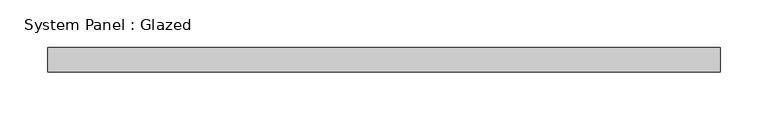
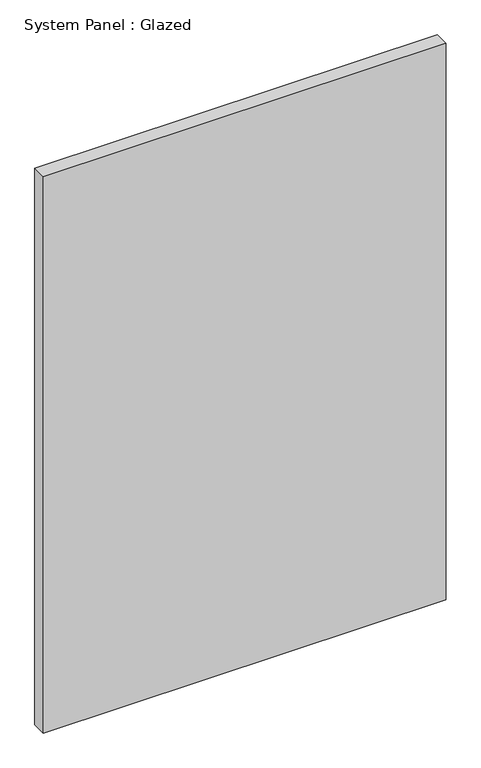
"""IFC4 building model written with IfcOpenShell, lengths in millimetres: plate geometry, System Panel : Glazed."""

from ifc_helpers import new_model, si_unit, origin, origin_with_axes, place, context, project, spatial, polyline, outline, extrude, source, transform, mapped, element, save


def system_panel_glazed_8af8589b(model_context):
    return source(origin(), model_context, "Body", "SweptSolid", [
        extrude(outline(polyline([(350.3083333, 19.05), (-350.3083333, 19.05), (-350.3083333, 44.45), (350.3083333, 44.45), (350.3083333, 19.05)])), origin_with_axes(), (0.0, 0.0, 1.0), 1022.35),
    ])


if __name__ == "__main__":
    model = new_model("IFC4")
    model_context = context("Model", 3, world=origin())
    ifc_project = project(units=[si_unit("LENGTHUNIT", "METRE", prefix="MILLI")], contexts=[model_context])
    site = spatial("IfcSite", under=ifc_project)
    building = spatial("IfcBuilding", under=site)
    placement = place(None, origin())
    system_panel_glazed_shape = system_panel_glazed_8af8589b(model_context)
    element("IfcPlate", 1, ObjectType="System Panel : Glazed", at=placement, inside=building, context=model_context, shape_type="MappedRepresentation", body=[
        mapped(system_panel_glazed_shape, transform((0.0, 0.0, 0.0), x_axis=(1.0, 0.0, 0.0), y_axis=(0.0, 1.0, 0.0), z_axis=(0.0, 0.0, 1.0))),
    ])
    save(model, "model.ifc")

# Revit data of these elements
# Type "System Panel : Glazed"
#   Construction Type Id = "GSP4R"
#   Analytic Construction = "1/8 in Pilkington single glazing"
#   Visual Light Transmittance = 0.9
#   Solar Heat Gain Coefficient = 0.86
#   Heat Transfer Coefficient (U) = 1.18115 BTU/(h·ft²·°F)
# Element 1 (IfcPlate, "System Panel : Glazed")
#   Materials on its faces: "Glass"
# Materials
#   "Glass": class "Glass", colour RGB 0 128 192, transparency 0.75, Description = "Soda Lime Glass", Cost = 0
